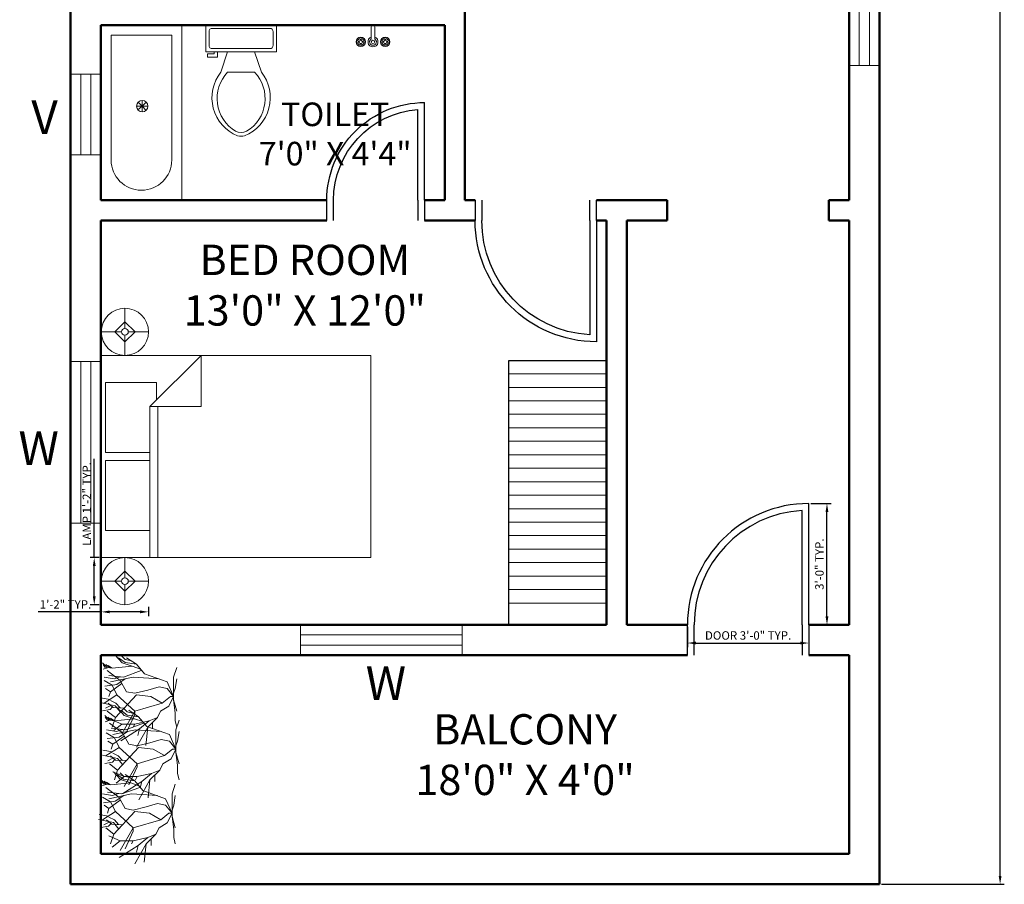
# Model space of a CAD drawing. Units: inches. Extents: x 995 to 2141, y 2161 to 2928.
# Tile 2 of 7: x 1418 to 1710, y 2281 to 2537. Entities that reach past the tile are written whole.
import ezdxf

# ---------------------------------------------------------------- set-up
doc = ezdxf.new("R2010")
doc.units = ezdxf.units.IN
for name, color, linetype, lineweight in [('A-ANNO-DIMS', 2, 'Continuous', 18), ('A-ANNO-TEXT', 7, 'Continuous', 18), ('A-AREA-IDEN', 7, 'Continuous', 25), ('A-DOOR', 3, 'Continuous', 25), ('A-FLOR-CASE', 8, 'Continuous', 25), ('A-FLOR-CASE-PATT', 252, 'Continuous', 13), ('A-FLOR-FIXT', 9, 'Continuous', 18), ('A-FURN', 8, 'Continuous', 18), ('A-GLAZ', 4, 'Continuous', 18), ('A-WALL', 7, 'Continuous', 50), ('L-PLNT-TREE', 94, 'Continuous', 13)]:
    doc.layers.add(name, color=color, linetype=linetype, lineweight=lineweight)
doc.styles.get("Standard").update_dxf_attribs({"font": 'arial.ttf'})
doc.dimstyles.new('ISO-25', dxfattribs={"dimtxt": 2.5, "dimasz": 2.5, "dimexe": 1.25, "dimexo": 0.625, "dimtad": 1, "dimdec": 0, "dimlunit": 3, "dimtxsty": 'Standard', "dimcen": 2.5, "dimadec": 0, "dimazin": 0, "dimtfac": 1, "dimtdec": 0, "dimtmove": 0, "dimatfit": 3, "dimfxl": 1, "dimarcsym": 0})

# ---------------------------------------------------------------- blocks, each defined once
blk = doc.blocks.new('Bed - Queen')
for p, q in [((0, -80.00003), (0, 0)), ((0, 0), (59.99999, 0)), ((59.99999, 0), (59.99999, -80.00003)), ((7.99999, -1.2), (28.79998, -1.2)), ((7.99999, -14.4), (7.99999, -1.2)), ((28.79998, -1.2), (28.79998, -14.4)), ((31.19999, -1.2), (51.99999, -1.2)), ((31.19999, -14.4), (31.19999, -1.2)), ((51.99999, -1.2), (51.99999, -16.4)), ((0, -14.4), (44.8, -14.4)), ((59.99999, -29.6), (44.8, -14.4)), ((44.8, -14.4), (44.8, -29.6)), ((44.8, -16.8), (0, -16.8)), ((51.99999, -16.4), (46.79936, -16.4)), ((44.8, -29.6), (59.99999, -29.6)), ((59.99999, -80.00003), (0, -80.00003))]:
    blk.add_line(p, q)
blk = doc.blocks.new('Lamp - Table')
for p, q in [((0, 7), (0, 1)), ((0, 3), (-3, 0)), ((3, 0), (0, 3)), ((-1, 0), (-7, 0)), ((-3, 0), (0, -3)), ((0, -3), (3, 0)), ((1, 0), (7, 0)), ((0, -1), (0, -7))]:
    blk.add_line(p, q)
for radius in [7, 1]:
    blk.add_circle((0, 0), radius)
blk = doc.blocks.new('Toilet - top')
for p, q in [((9.5, -6), (9.5, -2)), ((-10, -8.5), (-8, -8.5)), ((-10, -9.5), (-10, -8.5)), ((-8, -8.5), (-8, -8)), ((-7, -8), (-7, -9.5)), ((-4, -8), (-6, -14)), ((4, -8), (6, -14)), ((-7, -9.5), (-10, -9.5)), ((4, -14), (-4, -14))]:
    blk.add_line(p, q)
blk.add_lwpolyline([(10.5, -8), (10.5, 0), (-10.5, 0), (-10.5, -8)], close=True)
for points in [[(-9.5, -2), (-9.5, -6)], [(8.5, -1), (-8.5, -1)], [(-8.5, -7), (8.5, -7)]]:
    blk.add_lwpolyline(points)
for centre, radius, start, end in [((-8.62, -1.88), 0.884, 81.8699, 188.1301), ((8.62, -1.88), 0.884, 351.8699, 98.1301), ((-8.62, -6.12), 0.884, 171.8699, 278.1301), ((8.62, -6.12), 0.884, 261.8699, 8.1301), ((3.52, -21.58), 12.17, 141.4691, 247.9714), ((4.2, -21.82), 11.33, 136.3677, 238.9468), ((-3.52, -21.58), 12.17, 292.0284, 38.5307), ((-4.2, -21.82), 11.33, 301.053, 43.6321), ((0, -27.88), 4, 245.7318, 294.2682), ((0, -29), 4, 254.8605, 285.1395)]:
    blk.add_arc(centre, radius, start, end)
blk = doc.blocks.new('Faucet - Bathroom top')
for p, q in [((-4.107, 0.125), (-4.375, 0.125)), ((-3.75, 0.4788), (-3.75, 0.75)), ((-3.5, 0.482), (-3.5, 0.75)), ((-3.1461, 0.125), (-2.875, 0.125)), ((3.143, 0.125), (2.875, 0.125)), ((3.5, 0.4788), (3.5, 0.75)), ((3.75, 0.482), (3.75, 0.75)), ((4.1039, 0.125), (4.375, 0.125)), ((-4.1039, -0.125), (-4.375, -0.125)), ((-3.75, -0.4821), (-3.75, -0.75)), ((-3.5, -0.4789), (-3.5, -0.75)), ((-3.143, -0.125), (-2.875, -0.125)), ((-0.5, -0.8639), (-0.5, -4.5)), ((0.5, -4.5), (0.5, -0.8631)), ((3.1461, -0.125), (2.875, -0.125)), ((3.5, -0.4821), (3.5, -0.75)), ((3.75, -0.4789), (3.75, -0.75)), ((4.107, -0.125), (4.375, -0.125))]:
    blk.add_line(p, q)
for centre, radius in [((-3.625, 0), 1.375), ((-4.625, 0), 0.2795), ((-3.625, 0), 0.5), ((-3.625, 1), 0.2795), ((-2.625, 0), 0.2795), ((0, 0), 0.5), ((3.625, 0), 1.375), ((2.625, 0), 0.2795), ((3.625, 0), 0.5), ((3.625, 1), 0.2795), ((4.625, 0), 0.2795), ((-3.625, -1), 0.2795), ((3.625, -1), 0.2795)]:
    blk.add_circle(centre, radius)
for centre, radius, start, end in [((-3.625, 0), 1, 105.2407, 164.2093), ((-3.625, 0), 1, 16.44125, 74.07887), ((0, 0), 1.5, 289.6514, 250.3603), ((0, 0), 1, 300.3431, 239.7554), ((3.625, 0), 1, 106.12, 164.0884), ((3.625, 0), 1, 16.23422, 73.90469), ((-3.625, 0), 1, 196.2342, 253.9047), ((-3.625, 0), 1, 286.12, 344.0884), ((3.625, 0), 1, 196.4413, 254.0789), ((3.625, 0), 1, 285.2407, 344.2093), ((0, -4.5), 0.5, 180, 0)]:
    blk.add_arc(centre, radius, start, end)
blk = doc.blocks.new('*U15')
for p, q in [((-14.88, 18.24), (-12.96, 20.64)), ((-12.471, 19.775), (-12.898, 22.044)), ((-11.28, 19.619), (-12.104, 21.184)), ((-11.433, 18.289), (-10.457, 22.749)), ((-8.16, 17.76), (-10.56, 21.6)), ((-9.48, 19.775), (-8.992, 22.592)), ((-7.2, 19.68), (-6.24, 21.12)), ((-5.086, 17.741), (-5.513, 21.34)), ((-5.28, 19.2), (-3.84, 21.6)), ((-3.84, 16.8), (-0.96, 20.64)), ((-3.377, 18.602), (-2.888, 21.575)), ((-0.508, 21.888), (-0.081, 20.558)), ((-0.203, 19.149), (0.102, 21.34)), ((-0.02, 20.01), (0.896, 21.105)), ((0.041, 20.714), (1.384, 22.044)), ((0.102, 21.34), (0.835, 21.888)), ((-16.8, 16.32), (-18.72, 18.72)), ((-14.88, 18.24), (-17.76, 19.2)), ((-16.8, 16.32), (-15.36, 19.68)), ((-8.16, 12), (-14.88, 18.24)), ((-13.325, 16.724), (-11.433, 18.289)), ((-12.96, 12.48), (-8.16, 17.76)), ((-11.677, 19.071), (-12.471, 19.775)), ((-12.043, 15.628), (-11.921, 18.836)), ((-11.982, 16.802), (-10.579, 18.054)), ((-11.921, 18.836), (-10.64, 20.401)), ((-10.579, 18.054), (-9.846, 19.697)), ((-7.2, 19.68), (-8.64, 20.16)), ((-8.16, 17.76), (-5.28, 19.2)), ((-4.8, 16.32), (-7.2, 19.68)), ((-3.377, 15.315), (-5.086, 17.819)), ((-2.88, 12.96), (-4.32, 19.68)), ((-2.766, 16.802), (-3.377, 18.602)), ((-2.88, 15.84), (-2.4, 20.16)), ((0.346, 13.203), (-0.203, 19.149)), ((-0.142, 19.384), (0.59, 20.401)), ((1.323, 16.254), (3.642, 18.289)), ((-18.24, 11.04), (-21.755, 16.655)), ((-12.96, 12.48), (-19.68, 16.32)), ((-13.92, 12.48), (-19.2, 14.88)), ((-16.8, 12.48), (-16.8, 16.32)), ((-7.68, 12.48), (-7.2, 14.88)), ((-7.2, 14.88), (-3.84, 16.8)), ((-0.96, 10.56), (-2.88, 15.84)), ((0.346, 13.203), (1.323, 16.254)), ((0.96, 12), (1.44, 15.36)), ((0.96, 12), (2.88, 14.88)), ((1.44, 15.36), (2.88, 17.28)), ((1.92, 13.44), (2.4, 15.36)), ((2.4, 15.36), (3.36, 16.32)), ((-17.76, 8.64), (-23.663, 11.961)), ((-16.8, 12.48), (-17.76, 12.96)), ((-15.84, 8.16), (-16.8, 12.48)), ((-12.96, 12.48), (-13.92, 12.48)), ((-10.56, 4.32), (-12.96, 12.48)), ((-8.64, 7.68), (-8.16, 12)), ((-6.72, 8.64), (-7.68, 12.48)), ((-3.36, 5.28), (-2.88, 12.96)), ((-1.92, 9.6), (0.96, 12)), ((-0.48, 10.8), (0.346, 13.203)), ((-17.76, 8.64), (-23.128, 9.222)), ((-18.24, 11.04), (-20.16, 11.52)), ((-15.84, 8.16), (-18.24, 11.04)), ((-4.32, 2.88), (-1.92, 9.6)), ((-16.32, 7.2), (-18.24, 7.2)), ((-14.88, 5.76), (-17.76, 8.64)), ((-14.88, 5.76), (-15.84, 8.16)), ((-10.56, 4.32), (-8.64, 7.68)), ((-5.76, 5.28), (-6.72, 8.64)), ((-12.96, 4.8), (-14.88, 5.76)), ((-11.52, 2.4), (-12.96, 4.8)), ((-8.64, 1.92), (-10.56, 4.32)), ((-6.24, 2.88), (-5.76, 5.28)), ((-15.84, 0.48), (-17.76, 0)), ((-13.44, 0.48), (-15.84, 0.48)), ((-9.6, 0.96), (-13.44, 0.48)), ((-9.6, 0.96), (-12.96, 0)), ((-8.64, 0.96), (-11.52, 2.4)), ((-9.6, 0.96), (-7.68, 0.96)), ((-8.64, 0.96), (-4.32, 2.88)), ((-8.64, 0.96), (-6.24, 2.88)), ((-8.64, 0.96), (-8.64, 1.92)), ((-8.64, 0.96), (-2.88, 0.96)), ((-7.68, 0.96), (-6.24, 0.48)), ((-6.24, 0.48), (-3.36, 0)), ((-2.88, 0.96), (0, 0))]:
    blk.add_line(p, q)
blk = doc.blocks.new('*D21')
at = {"layer": 'A-ANNO-DIMS', "color": 0, "lineweight": -2, "transparency": 16777216}
for p, q in [((1673.63, 2880.52), (1710.02, 2880.52)), ((1708.77, 2283.02), (1708.77, 2878.02)), ((1673.63, 2280.52), (1710.02, 2280.52))]:
    blk.add_line(p, q, dxfattribs=at)
at = {"layer": 'A-ANNO-DIMS', "color": 0, "transparency": 16777216}
for points in [[(1708.36, 2878.02), (1709.19, 2878.02), (1708.77, 2880.52)], [(1708.36, 2283.02), (1709.19, 2283.02), (1708.77, 2280.52)]]:
    blk.add_solid(points, dxfattribs=at)
at = {"layer": 'Defpoints', "color": 0, "transparency": 16777216}
for p in [(1673, 2880.52), (1708.77, 2880.52), (1673, 2280.52)]:
    blk.add_point(p, dxfattribs=at)
at = {"layer": 'A-ANNO-DIMS', "color": 0, "transparency": 16777216, "insert": (1703.04, 2580.52), "char_height": 2.5, "attachment_point": 5, "rotation": 90}
blk.add_mtext("{\\H4x;50'}", dxfattribs=at)
blk = doc.blocks.new('WIN-48IN')
for p, q in [((0, 48), (0, 0)), ((9, 48), (0, 48)), ((3, 48), (3, 0)), ((6, 0), (6, 48)), ((9, 0), (9, 48)), ((0, 0), (9, 0))]:
    blk.add_line(p, q)
blk = doc.blocks.new('VENT-24IN')
for p, q in [((24, 9), (0, 9)), ((0, 9), (0, 0)), ((24, 9), (24, 0)), ((24, 6), (0, 6)), ((0, 3), (24, 3)), ((0, 0), (24, 0))]:
    blk.add_line(p, q)
blk = doc.blocks.new('DOOR-29IN-6IN-JAMB')
for p, q in [((35, 29), (29, 29)), ((35, 27), (29, 27)), ((29, 0), (0, 0)), ((29, 2), (2.07, 2)), ((29, 2), (35, 2)), ((29, 0), (35, 0))]:
    blk.add_line(p, q)
for radius, end in [(29, 180), (27, 175.752)]:
    blk.add_arc((29, 0), radius, 90, end)
blk = doc.blocks.new('DOOR-36IN-SWING')
for p, q in [((36, 0), (36, 36)), ((34, 0), (34, 33.94))]:
    blk.add_line(p, q)
for radius, start in [(36, 90), (34, 93.3723)]:
    blk.add_arc((36, 0), radius, start, 180)
blk = doc.blocks.new('*D34')
at = {"layer": 'A-ANNO-DIMS', "color": 0, "lineweight": -2, "transparency": 16777216}
for p, q in [((1616, 2356.89), (1616, 2350.87)), ((1652, 2356.89), (1652, 2350.87)), ((1618.5, 2352.12), (1649.5, 2352.12))]:
    blk.add_line(p, q, dxfattribs=at)
at = {"layer": 'A-ANNO-DIMS', "color": 0, "transparency": 16777216}
for points in [[(1618.5, 2352.53), (1618.5, 2351.7), (1616, 2352.12)], [(1649.5, 2352.53), (1649.5, 2351.7), (1652, 2352.12)]]:
    blk.add_solid(points, dxfattribs=at)
at = {"layer": 'Defpoints', "color": 0, "transparency": 16777216}
for p in [(1616, 2357.52), (1652, 2357.52), (1652, 2352.12)]:
    blk.add_point(p, dxfattribs=at)
at = {"layer": 'A-ANNO-DIMS', "color": 0, "transparency": 16777216, "insert": (1634, 2354.04), "char_height": 2.5, "attachment_point": 5}
blk.add_mtext('DOOR 3\'-0" TYP.', dxfattribs=at)
blk = doc.blocks.new('*D35')
at = {"layer": 'A-ANNO-DIMS', "color": 0, "lineweight": -2, "transparency": 16777216}
for p, q in [((1652.63, 2393.52), (1658.65, 2393.52)), ((1657.4, 2360.02), (1657.4, 2391.02)), ((1652.63, 2357.52), (1658.65, 2357.52))]:
    blk.add_line(p, q, dxfattribs=at)
at = {"layer": 'A-ANNO-DIMS', "color": 0, "transparency": 16777216}
for points in [[(1656.99, 2391.02), (1657.82, 2391.02), (1657.4, 2393.52)], [(1656.99, 2360.02), (1657.82, 2360.02), (1657.4, 2357.52)]]:
    blk.add_solid(points, dxfattribs=at)
at = {"layer": 'Defpoints', "color": 0, "transparency": 16777216}
for p in [(1652, 2393.52), (1657.4, 2393.52), (1652, 2357.52)]:
    blk.add_point(p, dxfattribs=at)
at = {"layer": 'A-ANNO-DIMS', "color": 0, "transparency": 16777216, "insert": (1655.5, 2375.52), "char_height": 2.5, "attachment_point": 5, "rotation": 90}
blk.add_mtext('3\'-0" TYP.', dxfattribs=at)
blk = doc.blocks.new('*D40')
at = {"layer": 'A-ANNO-DIMS', "color": 0, "lineweight": -2, "transparency": 16777216}
for p, q in [((1440, 2377.47), (1440, 2406.83)), ((1441.48, 2377.47), (1438.75, 2377.47)), ((1440, 2365.97), (1440, 2374.97)), ((1441.48, 2363.47), (1438.75, 2363.47))]:
    blk.add_line(p, q, dxfattribs=at)
at = {"layer": 'A-ANNO-DIMS', "color": 0, "transparency": 16777216}
for points in [[(1439.58, 2374.97), (1440.42, 2374.97), (1440, 2377.47)], [(1439.58, 2365.97), (1440.42, 2365.97), (1440, 2363.47)]]:
    blk.add_solid(points, dxfattribs=at)
at = {"layer": 'Defpoints', "color": 0, "transparency": 16777216}
for p in [(1440, 2377.47), (1442.1, 2377.47), (1442.1, 2363.47)]:
    blk.add_point(p, dxfattribs=at)
at = {"layer": 'A-ANNO-DIMS', "color": 0, "transparency": 16777216, "insert": (1438.12, 2393.4), "char_height": 2.5, "attachment_point": 5, "rotation": 90}
blk.add_mtext('LAMP 1\'-2" TYP.', dxfattribs=at)
blk = doc.blocks.new('*D41')
at = {"layer": 'A-ANNO-DIMS', "color": 0, "lineweight": -2, "transparency": 16777216}
for p, q in [((1442.1, 2361.37), (1423.35, 2361.37)), ((1442.1, 2362.84), (1442.1, 2360.12)), ((1453.6, 2361.37), (1444.6, 2361.37)), ((1456.1, 2362.84), (1456.1, 2360.12))]:
    blk.add_line(p, q, dxfattribs=at)
at = {"layer": 'A-ANNO-DIMS', "color": 0, "transparency": 16777216}
for points in [[(1444.6, 2361.78), (1444.6, 2360.95), (1442.1, 2361.37)], [(1453.6, 2361.78), (1453.6, 2360.95), (1456.1, 2361.37)]]:
    blk.add_solid(points, dxfattribs=at)
at = {"layer": 'Defpoints', "color": 0, "transparency": 16777216}
for p in [(1442.1, 2363.47), (1456.1, 2363.47), (1442.1, 2361.37)]:
    blk.add_point(p, dxfattribs=at)
at = {"layer": 'A-ANNO-DIMS', "color": 0, "transparency": 16777216, "insert": (1431.47, 2363.25), "char_height": 2.5, "attachment_point": 5}
blk.add_mtext('1\'-2" TYP.', dxfattribs=at)

msp = doc.modelspace()

# ---------------------------------------------------------------- hatches: boundary and pattern name
at = {"layer": 'A-FLOR-CASE-PATT'}
h = msp.add_hatch(dxfattribs=at)
h.set_pattern_fill('ANSI31', color=256, scale=1.259836, angle=-45, style=0)
h.paths.add_polyline_path([(1563, 2361.99), (1592, 2361.99), (1592, 2433.99), (1563, 2433.99)])

# ---------------------------------------------------------------- linework, layer by layer
at = {"layer": 'A-DOOR'}
for p, q in [((1553, 2483.52), (1553, 2477.52)), ((1555, 2483.52), (1555, 2477.52)), ((1587, 2477.52), (1587, 2483.52)), ((1589, 2477.52), (1589, 2483.52)), ((1616, 2348.52), (1616, 2357.52)), ((1618, 2348.52), (1618, 2357.52)), ((1650, 2357.52), (1650, 2348.52)), ((1652, 2357.52), (1652, 2348.52))]:
    msp.add_line(p, q, dxfattribs=at)
at = {"layer": 'A-FLOR-CASE'}
for p, q in [((1563, 2357.52), (1563, 2435.99)), ((1563, 2435.99), (1592, 2435.99))]:
    msp.add_line(p, q, dxfattribs=at)
at = {"layer": 'A-FLOR-FIXT'}
for p, q in [((1466, 2483.52), (1466, 2535.52)), ((1445, 2495.49), (1445, 2532.52)), ((1445, 2532.52), (1463, 2532.52)), ((1463, 2495.49), (1463, 2532.52)), ((1454.26, 2511.43), (1453.04, 2512.58)), ((1453.04, 2512.58), (1454.25, 2511.42)), ((1454.26, 2511.43), (1454.26, 2513.11)), ((1454.26, 2513.11), (1454.26, 2509.75)), ((1454.26, 2511.43), (1455.43, 2512.64)), ((1455.43, 2512.64), (1454.26, 2511.43)), ((1454.26, 2511.43), (1452.58, 2511.43)), ((1452.58, 2511.43), (1454.26, 2511.43)), ((1454.26, 2511.43), (1452.96, 2510.37)), ((1452.96, 2510.37), (1454.26, 2511.43)), ((1454.25, 2511.42), (1455.41, 2510.2)), ((1454.26, 2509.75), (1454.26, 2511.43)), ((1454.26, 2511.43), (1455.94, 2511.43)), ((1455.94, 2511.43), (1454.26, 2511.43)), ((1453.29, 2486.52), (1454.72, 2486.52))]:
    msp.add_line(p, q, dxfattribs=at)
msp.add_circle((1454.26, 2511.43), 1.68, dxfattribs=at)
msp.add_arc((1454, 2495.49), 9, 180, 0, dxfattribs=at)
at = {"layer": 'A-WALL'}
for p, q in [((1433, 2280.52), (1433, 2880.52)), ((1673, 2880.52), (1673, 2280.52)), ((1664, 2709.52), (1664, 2483.52)), ((1550, 2535.52), (1550, 2541.52)), ((1442, 2535.52), (1544, 2535.52)), ((1442, 2483.52), (1442, 2535.52)), ((1544, 2483.52), (1544, 2535.52)), ((1550, 2483.52), (1550, 2535.52)), ((1442, 2483.52), (1509, 2483.52)), ((1544, 2483.52), (1538, 2483.52)), ((1538, 2483.52), (1544, 2483.52)), ((1550, 2483.52), (1553, 2483.52)), ((1553, 2483.52), (1550, 2483.52)), ((1589, 2483.52), (1610, 2483.52)), ((1610, 2477.52), (1610, 2483.52)), ((1658, 2483.52), (1658, 2477.52)), ((1658, 2477.52), (1658, 2483.52)), ((1658, 2483.52), (1664, 2483.52)), ((1442, 2477.52), (1509, 2477.52)), ((1442, 2357.52), (1442, 2477.52)), ((1538, 2477.52), (1553, 2477.52)), ((1550, 2477.52), (1553, 2477.52)), ((1592, 2477.52), (1589, 2477.52)), ((1592, 2477.52), (1589, 2477.52)), ((1589, 2477.52), (1592, 2477.52)), ((1592, 2357.52), (1592, 2477.52)), ((1598, 2357.52), (1598, 2477.52)), ((1598, 2477.52), (1610, 2477.52)), ((1598, 2477.52), (1610, 2477.52)), ((1658, 2477.52), (1664, 2477.52)), ((1664, 2477.52), (1664, 2357.52)), ((1442, 2357.52), (1592, 2357.52)), ((1598, 2357.52), (1616, 2357.52)), ((1664, 2357.52), (1652, 2357.52)), ((1652, 2357.52), (1664, 2357.52)), ((1442, 2289.52), (1442, 2348.52)), ((1442, 2348.52), (1592, 2348.52)), ((1598, 2348.52), (1592, 2348.52)), ((1598, 2348.52), (1616, 2348.52)), ((1652, 2348.52), (1664, 2348.52)), ((1664, 2348.52), (1664, 2289.52)), ((1664, 2289.52), (1442, 2289.52)), ((1673, 2280.52), (1433, 2280.52))]:
    msp.add_line(p, q, dxfattribs=at)

# ---------------------------------------------------------------- block references
at = {"layer": 'A-DOOR', "extrusion": (0, 0, -1), "zscale": -1}
for name, p, rotation in [('DOOR-29IN-6IN-JAMB', (-1538, 2512.52), 270.0000000000022), ('DOOR-36IN-SWING', (-1553, 2477.52), 180)]:
    msp.add_blockref(name, p, dxfattribs=dict(at, rotation=rotation))
at = {"layer": 'A-DOOR'}
msp.add_blockref('DOOR-36IN-SWING', (1616, 2357.52), dxfattribs=at)
at = {"layer": 'A-FLOR-FIXT'}
msp.add_blockref('Toilet - top', (1483.58, 2535.52), dxfattribs=at)
at = {"layer": 'A-FLOR-FIXT', "rotation": 180}
msp.add_blockref('Faucet - Bathroom top', (1522.71, 2530.52), dxfattribs=at)
at = {"layer": 'A-FURN', "rotation": 89.99999999999999}
for name, p in [('Lamp - Table', (1449.1, 2444.47)), ('Bed - Queen', (1442.1, 2377.47)), ('Lamp - Table', (1449.1, 2370.47))]:
    msp.add_blockref(name, p, dxfattribs=at)
at = {"layer": 'A-GLAZ'}
for p in [(1664, 2523.48), (1433, 2387.7)]:
    msp.add_blockref('WIN-48IN', p, dxfattribs=at)
for name, p, rotation in [('VENT-24IN', (1442, 2496.98), 89.99999999999966), ('WIN-48IN', (1549.17, 2348.52), 90.00000000000104)]:
    msp.add_blockref(name, p, dxfattribs=dict(at, rotation=rotation))
at = {"layer": 'L-PLNT-TREE', "rotation": 90}
for p in [(1464.5, 2344.88), (1465.18, 2329.27), (1464.05, 2310.25)]:
    msp.add_blockref('*U15', p, dxfattribs=at)

# ---------------------------------------------------------------- texts
at = {"layer": 'A-ANNO-TEXT', "char_height": 10, "attachment_point": 1}
for s, insert in [('V', (1421.33, 2513.17)), ('W', (1417.53, 2414.91)), ('W', (1520.55, 2345.19))]:
    msp.add_mtext_dynamic_manual_height_columns(s, width=112.484, gutter_width=12.5, heights=[0], dxfattribs=dict(at, insert=insert))
at = {"layer": 'A-AREA-IDEN', "attachment_point": 1}
for s, width, insert, char_height in [('\\pxqc;TOILET\\P7\'0" X 4\'4"', 53.0246, (1484.98, 2512.52), 7), ('\\pxqc;BED ROOM ^J13\'0" X 12\'0"', 109.7687, (1447.6, 2470.32), 9), ('\\pxqc;BALCONY \\P18\'0" X 4\'0"', 118.2971, (1508.7, 2331.01), 9)]:
    msp.add_mtext_dynamic_manual_height_columns(s, width=width, gutter_width=12.5, heights=[0], dxfattribs=dict(at, insert=insert, char_height=char_height))

# ---------------------------------------------------------------- dimensions: what is measured, and where the dimension line sits
at = {"layer": 'A-ANNO-DIMS'}
for base, p1, p2, angle, text, override, picture, middle in [((1708.77, 2880.52), (1673, 2280.52), (1673, 2880.52), 90, "{\\H4x;50'}", {"dimclrd": 0, "dimclre": 0, "dimclrt": 0}, '*D21', (1703.04, 2580.52)), ((1440, 2377.47), (1442.1, 2363.47), (1442.1, 2377.47), 90, 'LAMP <> TYP.', {"dimdec": 1, "dimlfac": 1, "dimrnd": 0, "dimzin": 1, "dimdsep": 46, "dimlunit": 4, "dimfrac": 2}, '*D40', (1438.12, 2393.4)), ((1657.4, 2393.52), (1652, 2357.52), (1652, 2393.52), 90, '<> TYP.', {"dimdec": 1, "dimlfac": 1, "dimrnd": 0, "dimzin": 1, "dimdsep": 46, "dimlunit": 4, "dimfrac": 2}, '*D35', (1655.5, 2375.52)), ((1442.1, 2361.37), (1456.1, 2363.47), (1442.1, 2363.47), 180, '<> TYP.', {"dimdec": 1, "dimlfac": 1, "dimrnd": 0, "dimzin": 1, "dimdsep": 46, "dimlunit": 4, "dimfrac": 2}, '*D41', (1431.47, 2363.25))]:
    dim = msp.add_linear_dim(base=base, p1=p1, p2=p2, angle=angle, text=text, dimstyle='ISO-25', override=override, dxfattribs=at)
    dim.commit()
    dim.dimension.update_dxf_attribs({"geometry": picture, "text_midpoint": middle})
dim = msp.add_linear_dim(base=(1652, 2352.12), p1=(1616, 2357.52), p2=(1652, 2357.52), text='DOOR <> TYP.', dimstyle='ISO-25', override={"dimdec": 1, "dimlfac": 1, "dimrnd": 0, "dimzin": 1, "dimdsep": 46, "dimlunit": 4, "dimfrac": 2}, dxfattribs=at)
dim.commit()
dim.dimension.update_dxf_attribs({"geometry": '*D34', "text_midpoint": (1634, 2354.04)})

doc.saveas('drawing.dxf')
